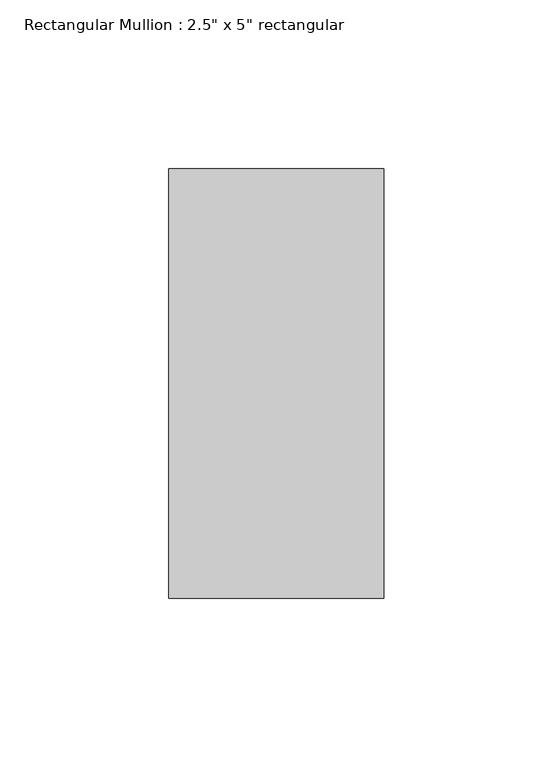
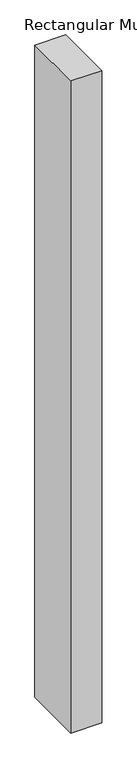
"""IFC4 building model written with IfcOpenShell, lengths in millimetres: member geometry."""

from ifc_helpers import new_model, si_unit, frame, origin, place, context, project, spatial, polyline, outline, extrude, source, transform, mapped, element, save


def member_b1264396(model_context):
    return source(origin(), model_context, "Body", "SweptSolid", [
        extrude(outline(polyline([(31.75, 63.5), (31.75, -63.5), (-31.75, -63.5), (-31.75, 63.5), (31.75, 63.5)])), frame((0.0, 0.0, -1408.8373989), z_axis=(0.0, 0.0, 1.0), x_axis=(1.0, 0.0, 0.0)), (0.0, 0.0, 1.0), 1408.8373989),
    ])


if __name__ == "__main__":
    model = new_model("IFC4")
    model_context = context("Model", 3, world=origin())
    ifc_project = project(units=[si_unit("LENGTHUNIT", "METRE", prefix="MILLI")], contexts=[model_context])
    site = spatial("IfcSite", under=ifc_project)
    building = spatial("IfcBuilding", under=site)
    placement = place(None, origin())
    member_shape = member_b1264396(model_context)
    element("IfcMember", 1, ObjectType="Rectangular Mullion : 2.5\" x 5\" rectangular", at=placement, inside=building, context=model_context, shape_type="MappedRepresentation", body=[
        mapped(member_shape, transform((0.0, 0.0, 0.0), x_axis=(1.0, 0.0, 0.0), y_axis=(0.0, 1.0, 0.0), z_axis=(0.0, 0.0, 1.0))),
    ])
    save(model, "model.ifc")

# Revit data of these elements
# Type "Rectangular Mullion : 2.5\" x 5\" rectangular"
#   built-in parameter 1007304 = 0.416667 (stored number, unit not read)
#   built-in parameter 1007301 = 0.104167 (stored number, unit not read)
#   built-in parameter 1007300 = 0.104167 (stored number, unit not read)
# Element 1 (IfcMember, "Rectangular Mullion : 2.5\" x 5\" rectangular")
#   Materials on its faces: "Aluminum"
# Materials
#   "Aluminum": class "Metal", colour RGB 247 247 247, transparency 0, Description = "Aluminum 6061", Cost = 0
